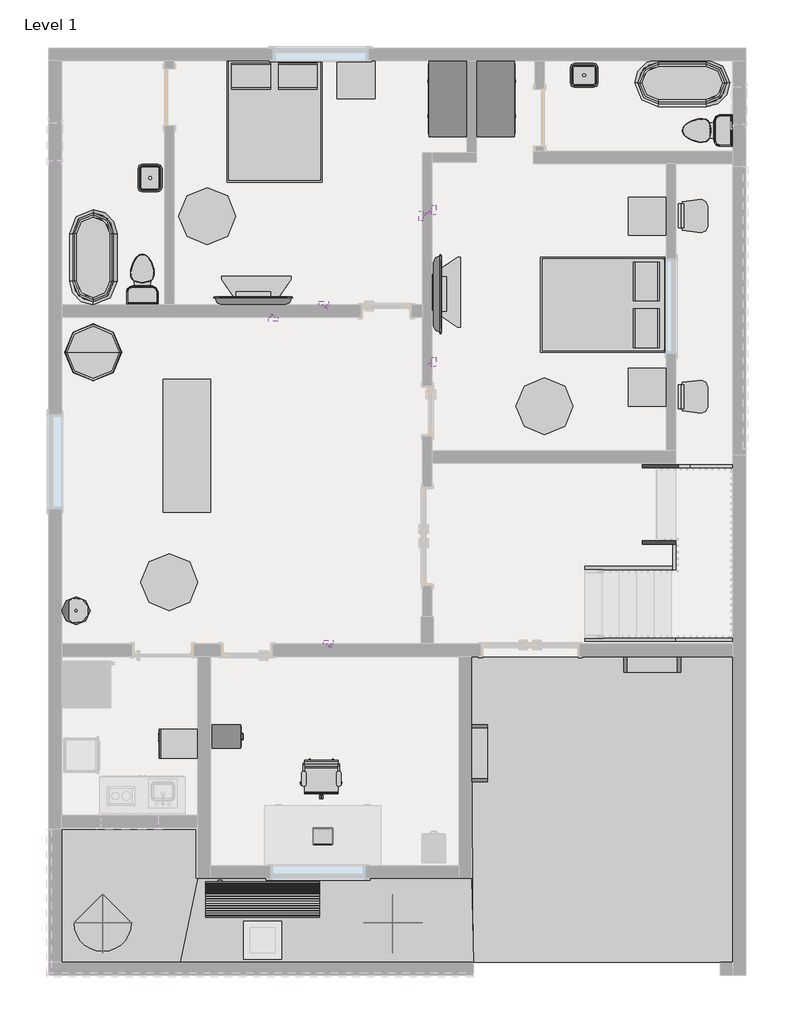
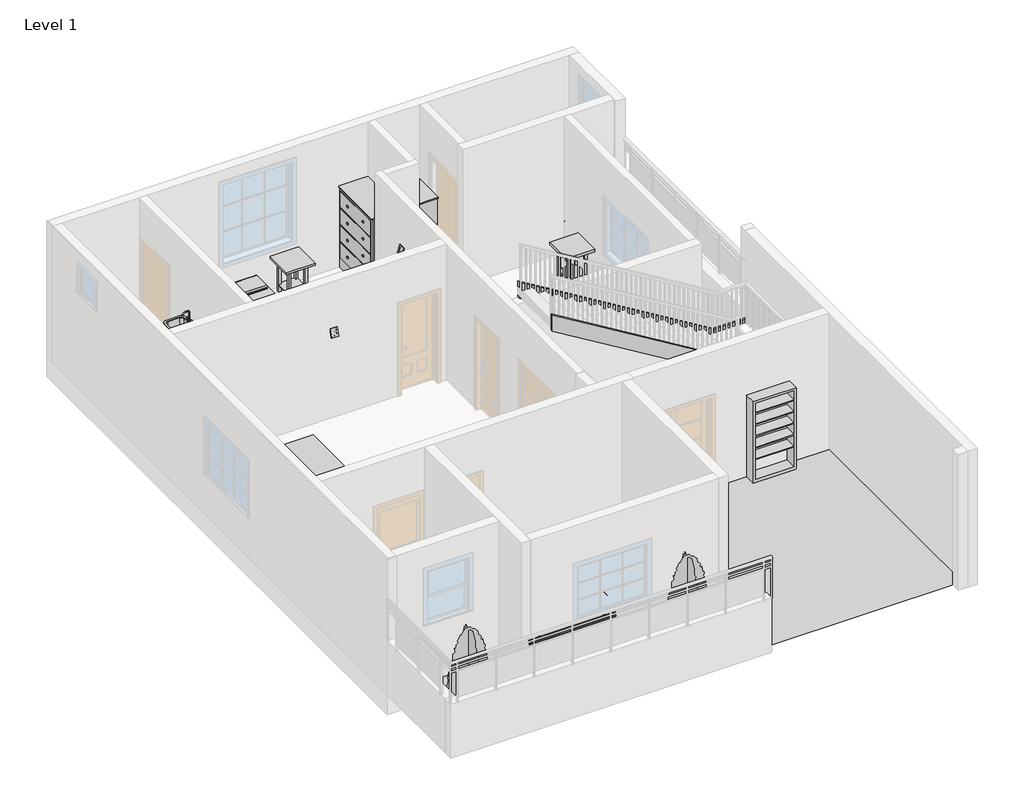
# One storey, part 4 of 4: 22 furniture elements, 11 proxies, 8 members, 7 flow terminals, 3 geographic elements.
"""IFC4 building model written with IfcOpenShell, lengths in millimetres."""

from ifc_helpers import new_model, si_unit, frame, origin, place, context, project, spatial, polyline, outline, extrude, faceted_brep, triangles, transform, mapped, element, save
from components import entourage_4c8cfd20, proxy_7e1014cc, rpc_picture_frame_rpc_picture_frame_c25e3fe9, flow_terminal_d49f872f, flow_terminal_62a433f7, toilet_domestic_3d_toilet_domestic_3d_f7549cf7, toilet_domestic_3d_toilet_domestic_3d_183bbd19, flow_terminal_b374fae2, furniture_1d2926bd, furniture_d4d3357e, chair_desk_chair_desk_ccc35c8f, chair_task_arms_chair_task_arms_fa5a08ef, furniture_9fa109b2, furniture_417d203a, furniture_fdf74506, tv_stand_tv_stand_6ce107e5, furniture_92191dda, furniture_905aceb5, furniture_4bee3317, furniture_5bc9ed15, furniture_c80d6d9c, geographic_element_235d1464, rpc_tree_conifer_chinese_juniper_7_1b9786cd

model = new_model("IFC4")

# Units and contexts
model_context = context("Model", 3, world=origin())
ifc_project = project(units=[si_unit("LENGTHUNIT", "METRE", prefix="MILLI")], contexts=[model_context])

# Site, building, storey
site = spatial("IfcSite", under=ifc_project)
building = spatial("IfcBuilding", under=site)
storey = spatial("IfcBuildingStorey", under=building, Name="Level 1", Elevation=0.0)

# Proxies
placement = place(None, origin())
element("IfcBuildingElementProxy", 1, Name="Building Element Proxy", at=placement, inside=storey, context=model_context, shape_type="Tessellation", body=[
    triangles([(-4983.3888428, 2180.3574657, 0.0), (-792.3886248, 2180.3574657, 0.0), (-792.3886248, -2721.8425827, 0.0), (-4957.988649, -2721.8425827, 0.0)], [[1, 4, 2], [3, 2, 4]], closed=False),
])
element("IfcBuildingElementProxy", 2, Name="Building Element Proxy", at=placement, inside=storey, context=model_context, shape_type="Tessellation", body=[
    triangles([(-11561.9884552, -588.24251, 0.0), (-9377.588649, -562.8424979, 0.0), (-9377.588649, -1375.6424858, 0.0), (-11561.9884552, -2721.8425827, 0.0), (-9661.5468979, -2721.8425827, 0.0)], [[1, 4, 3], [3, 2, 1], [3, 4, 5]], closed=False),
])
element("IfcBuildingElementProxy", 3, Name="Building Element Proxy", at=placement, inside=storey, context=model_context, shape_type="Tessellation", body=[
    triangles([(-9657.6913193, -2721.8425827, 0.0), (-9377.588649, -1375.6424858, 0.0), (-4983.3888428, -1375.6424858, 0.0), (-4957.988649, -2721.8425827, 0.0)], [[2, 1, 4], [4, 3, 2]], closed=False),
])
entourage_shape = entourage_4c8cfd20(model_context)
element("IfcBuildingElementProxy", 4, Name="Entourage", at=placement, inside=storey, context=model_context, shape_type="MappedRepresentation", body=[
    mapped(entourage_shape, transform((-7370.5830981, -664.4425054, 762.0), x_axis=(1.0, 0.0, 0.0), y_axis=(0.0, 1.0, 0.0), z_axis=(0.0, 0.0, 1.0))),
])
proxy_shape = proxy_7e1014cc(model_context)
element("IfcBuildingElementProxy", 5, Name="18\" x 24\" x 34 1/2\"", ObjectType="18\" x 24\" x 34 1/2\"", at=placement, inside=storey, context=model_context, shape_type="MappedRepresentation", body=[
    mapped(proxy_shape, transform((-9948.8381931, 1089.4749631, 0.0), x_axis=(0.0, -1.0, 0.0), y_axis=(1.0, 0.0, 0.0), z_axis=(0.0, 0.0, 1.0))),
])
rpc_picture_frame_rpc_picture_frame_shape = rpc_picture_frame_rpc_picture_frame_c25e3fe9(model_context)
element("IfcBuildingElementProxy", 6, Name="RPC Picture Frame : RPC Picture Frame", ObjectType="RPC Picture Frame : RPC Picture Frame", at=placement, inside=storey, context=model_context, shape_type="MappedRepresentation", body=[
    mapped(rpc_picture_frame_rpc_picture_frame_shape, transform((-7352.9458894, 7819.1574946, 1828.8), x_axis=(-0.9999999999999998, 0.0, 0.0), y_axis=(0.0, -0.9999999999999998, 0.0), z_axis=(0.0, 0.0, 1.0))),
])
element("IfcBuildingElementProxy", 7, Name="RPC Picture Frame : RPC Picture Frame", ObjectType="RPC Picture Frame : RPC Picture Frame", at=placement, inside=storey, context=model_context, shape_type="MappedRepresentation", body=[
    mapped(rpc_picture_frame_rpc_picture_frame_shape, transform((-5770.7886283, 9241.5574946, 1828.8), x_axis=(0.0, -1.0000000000000002, 0.0), y_axis=(1.0000000000000002, 0.0, 0.0), z_axis=(0.0, 0.0, 1.0))),
])
element("IfcBuildingElementProxy", 8, Name="RPC Picture Frame : RPC Picture Frame", ObjectType="RPC Picture Frame : RPC Picture Frame", at=placement, inside=storey, context=model_context, shape_type="MappedRepresentation", body=[
    mapped(rpc_picture_frame_rpc_picture_frame_shape, transform((-5618.3886283, 9336.9494679, 1828.8), x_axis=(0.0, 1.0000000000000004, 0.0), y_axis=(-1.0000000000000004, 0.0, 0.0), z_axis=(0.0, 0.0, 1.0))),
])
element("IfcBuildingElementProxy", 9, Name="RPC Picture Frame : RPC Picture Frame", ObjectType="RPC Picture Frame : RPC Picture Frame", at=placement, inside=storey, context=model_context, shape_type="MappedRepresentation", body=[
    mapped(rpc_picture_frame_rpc_picture_frame_shape, transform((-5618.3886283, 6905.8954271, 1828.8), x_axis=(0.0, 1.0000000000000002, 0.0), y_axis=(-1.0000000000000002, 0.0, 0.0), z_axis=(0.0, 0.0, 1.0))),
])
element("IfcBuildingElementProxy", 10, Name="RPC Picture Frame : RPC Picture Frame", ObjectType="RPC Picture Frame : RPC Picture Frame", at=placement, inside=storey, context=model_context, shape_type="MappedRepresentation", body=[
    mapped(rpc_picture_frame_rpc_picture_frame_shape, transform((-7281.3925432, 2383.5574946, 1828.8), x_axis=(-1.0, 0.0, 0.0), y_axis=(0.0, -1.0, 0.0), z_axis=(0.0, 0.0, 1.0))),
])
element("IfcBuildingElementProxy", 11, Name="RPC Picture Frame : RPC Picture Frame", ObjectType="RPC Picture Frame : RPC Picture Frame", at=placement, inside=storey, context=model_context, shape_type="MappedRepresentation", body=[
    mapped(rpc_picture_frame_rpc_picture_frame_shape, transform((-8165.6222602, 7615.9574946, 1828.8), x_axis=(1.0000000000000002, 0.0, 0.0), y_axis=(0.0, 1.0000000000000002, 0.0), z_axis=(0.0, 0.0, 1.0))),
])

# Flow terminals
flow_terminal_shape = flow_terminal_d49f872f(model_context)
element("IfcFlowTerminal", 12, ObjectType="Sink Vanity-Round : 19\" x 19\"", at=placement, inside=storey, context=model_context, shape_type="MappedRepresentation", body=[
    mapped(flow_terminal_shape, transform((-11245.3762507, 2820.305754, 457.2), x_axis=(0.0, 1.0000000000000002, 0.0), y_axis=(-1.0000000000000002, 0.0, 0.0), z_axis=(0.0, 0.0, 1.0))),
])
flow_terminal_2_shape = flow_terminal_62a433f7(model_context)
element("IfcFlowTerminal", 13, ObjectType="Sink Vanity-Square : 20\" x 18\"", at=placement, inside=storey, context=model_context, shape_type="MappedRepresentation", body=[
    mapped(flow_terminal_2_shape, transform((-3195.6778689, 11550.6120935, 609.6), x_axis=(1.0, 0.0, 0.0), y_axis=(0.0, 1.0, 0.0), z_axis=(0.0, 0.0, 1.0))),
])
element("IfcFlowTerminal", 14, ObjectType="Sink Vanity-Square : 20\" x 18\"", at=placement, inside=storey, context=model_context, shape_type="MappedRepresentation", body=[
    mapped(flow_terminal_2_shape, transform((-10091.1340294, 9866.8467351, 609.6), x_axis=(0.0, -1.0, 0.0), y_axis=(1.0, 0.0, 0.0), z_axis=(0.0, 0.0, 1.0))),
])
toilet_domestic_3d_toilet_domestic_3d_shape = toilet_domestic_3d_toilet_domestic_3d_f7549cf7(model_context)
toilet_domestic_3d_toilet_domestic_3d_2_shape = toilet_domestic_3d_toilet_domestic_3d_183bbd19(model_context)
element("IfcFlowTerminal", 15, ObjectType="Toilet-Domestic-3D : Toilet-Domestic-3D", at=placement, inside=storey, context=model_context, shape_type="MappedRepresentation", body=[
    mapped(toilet_domestic_3d_toilet_domestic_3d_shape, transform((-1300.3886283, 10613.1574946, 0.0), x_axis=(0.0, -1.0000000000000002, 0.0), y_axis=(1.0000000000000002, 0.0, 0.0), z_axis=(0.0, 0.0, 1.0))),
    mapped(toilet_domestic_3d_toilet_domestic_3d_2_shape, transform((-1300.3886283, 10613.1574946, 0.0), x_axis=(0.0, -1.0000000000000002, 0.0), y_axis=(1.0000000000000002, 0.0, 0.0), z_axis=(0.0, 0.0, 1.0))),
])
element("IfcFlowTerminal", 16, ObjectType="Toilet-Domestic-3D : Toilet-Domestic-3D", at=placement, inside=storey, context=model_context, shape_type="MappedRepresentation", body=[
    mapped(toilet_domestic_3d_toilet_domestic_3d_shape, transform((-10266.5886283, 8327.1574946, 0.0), x_axis=(-0.9999999999999998, 0.0, 0.0), y_axis=(0.0, -0.9999999999999998, 0.0), z_axis=(0.0, 0.0, 1.0))),
    mapped(toilet_domestic_3d_toilet_domestic_3d_2_shape, transform((-10266.5886283, 8327.1574946, 0.0), x_axis=(-0.9999999999999998, 0.0, 0.0), y_axis=(0.0, -0.9999999999999998, 0.0), z_axis=(0.0, 0.0, 1.0))),
])
flow_terminal_3_shape = flow_terminal_b374fae2(model_context)
element("IfcFlowTerminal", 17, ObjectType="Tub-Free Standing-3D : 30\" x 60\"", at=placement, inside=storey, context=model_context, shape_type="MappedRepresentation", body=[
    mapped(flow_terminal_3_shape, transform((-1605.1886283, 11375.1574946, 0.0), x_axis=(0.0, -1.0, 0.0), y_axis=(1.0, 0.0, 0.0), z_axis=(0.0, 0.0, 1.0))),
])
element("IfcFlowTerminal", 18, ObjectType="Tub-Free Standing-3D : 30\" x 60\"", at=placement, inside=storey, context=model_context, shape_type="MappedRepresentation", body=[
    mapped(flow_terminal_3_shape, transform((-11053.9886283, 8581.1574946, 0.0), x_axis=(-1.0000000000000002, 0.0, 0.0), y_axis=(0.0, -1.0000000000000002, 0.0), z_axis=(0.0, 0.0, 1.0))),
])

# Furniture
furniture_shape = furniture_1d2926bd(model_context)
element("IfcFurniture", 19, ObjectType="Bed-Box : Queen 60\" x 79\"", at=placement, inside=storey, context=model_context, shape_type="MappedRepresentation", body=[
    mapped(furniture_shape, transform((-2640.7591201, 8158.3099536, 0.0), x_axis=(0.0, -1.0, 0.0), y_axis=(1.0, 0.0, 0.0), z_axis=(0.0, 0.0, 1.0))),
])
element("IfcFurniture", 20, ObjectType="Bed-Box : Queen 60\" x 79\"", at=placement, inside=storey, context=model_context, shape_type="MappedRepresentation", body=[
    mapped(furniture_shape, transform((-8484.8410873, 11025.3870028, 0.0), x_axis=(1.0, 0.0, 0.0), y_axis=(0.0, 1.0, 0.0), z_axis=(0.0, 0.0, 1.0))),
])
furniture_2_shape = furniture_d4d3357e(model_context)
element("IfcFurniture", 21, ObjectType="Cabinet-File 5 Drawer : 15\" x 18\"", at=placement, inside=storey, context=model_context, shape_type="MappedRepresentation", body=[
    mapped(furniture_2_shape, transform((-9062.5229284, 1025.5539416, 0.0), x_axis=(0.0, 1.0, 0.0), y_axis=(-1.0, 0.0, 0.0), z_axis=(0.0, 0.0, 1.0))),
])
chair_desk_chair_desk_shape = chair_desk_chair_desk_ccc35c8f(model_context)
element("IfcFurniture", 22, ObjectType="Chair-Desk : Chair-Desk", at=placement, inside=storey, context=model_context, shape_type="MappedRepresentation", body=[
    mapped(chair_desk_chair_desk_shape, transform((-1605.1886283, 6345.9574946, 0.0), x_axis=(0.0, -1.0000000000000007, 0.0), y_axis=(1.0000000000000007, 0.0, 0.0), z_axis=(0.0, 0.0, 1.0))),
])
element("IfcFurniture", 23, ObjectType="Chair-Desk : Chair-Desk", at=placement, inside=storey, context=model_context, shape_type="MappedRepresentation", body=[
    mapped(chair_desk_chair_desk_shape, transform((-1605.1886283, 9241.5574946, 0.0), x_axis=(0.0, -1.0000000000000002, 0.0), y_axis=(1.0000000000000002, 0.0, 0.0), z_axis=(0.0, 0.0, 1.0))),
])
chair_task_arms_chair_task_arms_shape = chair_task_arms_chair_task_arms_fa5a08ef(model_context)
element("IfcFurniture", 24, ObjectType="Chair-Task Arms : Chair-Task Arms", at=placement, inside=storey, context=model_context, shape_type="MappedRepresentation", body=[
    mapped(chair_task_arms_chair_task_arms_shape, transform((-7255.3978086, 268.9033962, 0.0), x_axis=(-0.9999999999999999, 0.0, 0.0), y_axis=(0.0, -0.9999999999999999, 0.0), z_axis=(0.0, 0.0, 1.0))),
])
furniture_3_shape = furniture_9fa109b2(model_context)
element("IfcFurniture", 25, ObjectType="Dresser : 48\" x 72\" x 24\"", at=placement, inside=storey, context=model_context, shape_type="MappedRepresentation", body=[
    mapped(furniture_3_shape, transform((-4965.5515824, 11390.3507544, 0.0), x_axis=(0.0, 1.0, 0.0), y_axis=(-1.0, 0.0, 0.0), z_axis=(0.0, 0.0, 1.0))),
])
element("IfcFurniture", 26, ObjectType="Dresser : 48\" x 72\" x 24\"", at=placement, inside=storey, context=model_context, shape_type="MappedRepresentation", body=[
    mapped(furniture_3_shape, transform((-5001.2256742, 10851.9642347, 0.0), x_axis=(0.0, -1.0000000000000007, 0.0), y_axis=(1.0000000000000007, 0.0, 0.0), z_axis=(0.0, 0.0, 1.0))),
])
furniture_4_shape = furniture_417d203a(model_context)
element("IfcFurniture", 27, ObjectType="Shelving : 36\" x 10\" x 72\"", at=placement, inside=storey, context=model_context, shape_type="MappedRepresentation", body=[
    mapped(furniture_4_shape, transform((-5161.1886283, 630.9574946, 0.0), x_axis=(0.0, 1.0, 0.0), y_axis=(-1.0, 0.0, 0.0), z_axis=(0.0, 0.0, 1.0))),
])
element("IfcFurniture", 28, ObjectType="Shelving : 36\" x 10\" x 72\"", at=placement, inside=storey, context=model_context, shape_type="MappedRepresentation", body=[
    mapped(furniture_4_shape, transform((-2087.7886283, 1748.5574946, 0.0), x_axis=(-1.0000000000000002, 0.0, 0.0), y_axis=(0.0, -1.0000000000000002, 0.0), z_axis=(0.0, 0.0, 1.0))),
])
furniture_5_shape = furniture_fdf74506(model_context)
element("IfcFurniture", 29, ObjectType="TV - Flat Screen : 50\"", at=placement, inside=storey, context=model_context, shape_type="MappedRepresentation", body=[
    mapped(furniture_5_shape, transform((-8492.5331425, 7877.6961182, 914.4), x_axis=(-1.0000000000000002, 0.0, 0.0), y_axis=(0.0, -1.0000000000000002, 0.0), z_axis=(0.0, 0.0, 1.0))),
])
element("IfcFurniture", 30, ObjectType="TV - Flat Screen : 50\"", at=placement, inside=storey, context=model_context, shape_type="MappedRepresentation", body=[
    mapped(furniture_5_shape, transform((-5539.8500047, 7993.819929, 914.4), x_axis=(0.0, 1.0000000000000002, 0.0), y_axis=(-1.0000000000000002, 0.0, 0.0), z_axis=(0.0, 0.0, 1.0))),
])
tv_stand_tv_stand_shape = tv_stand_tv_stand_6ce107e5(model_context)
element("IfcFurniture", 31, ObjectType="TV Stand : TV Stand", at=placement, inside=storey, context=model_context, shape_type="MappedRepresentation", body=[
    mapped(tv_stand_tv_stand_shape, transform((-8312.6006262, 7819.1574946, 0.0), x_axis=(-1.0000000000000002, 0.0, 0.0), y_axis=(0.0, -1.0000000000000002, 0.0), z_axis=(0.0, 0.0, 1.0))),
])
element("IfcFurniture", 32, ObjectType="TV Stand : TV Stand", at=placement, inside=storey, context=model_context, shape_type="MappedRepresentation", body=[
    mapped(tv_stand_tv_stand_shape, transform((-5618.3886283, 7897.1694925, 0.0), x_axis=(0.0, 1.0, 0.0), y_axis=(-1.0, 0.0, 0.0), z_axis=(0.0, 0.0, 1.0))),
])
furniture_6_shape = furniture_92191dda(model_context)
element("IfcFurniture", 33, ObjectType="Table-Dining : 30\" x 84\" x 22\"", at=placement, inside=storey, context=model_context, shape_type="MappedRepresentation", body=[
    mapped(furniture_6_shape, transform((-9460.1775505, 5540.2917279, 0.0), x_axis=(0.0, 1.0, 0.0), y_axis=(-1.0, 0.0, 0.0), z_axis=(0.0, 0.0, 1.0))),
])
furniture_7_shape = furniture_905aceb5(model_context)
element("IfcFurniture", 34, ObjectType="Table-Dining Round w Chairs : 36\" Diameter", at=placement, inside=storey, context=model_context, shape_type="MappedRepresentation", body=[
    mapped(furniture_7_shape, transform((-9938.4705955, 3559.0361831, 0.0), x_axis=(1.0, 0.0, 0.0), y_axis=(0.0, 1.0, 0.0), z_axis=(0.0, 0.0, 1.0))),
])
furniture_8_shape = furniture_4bee3317(model_context)
element("IfcFurniture", 35, ObjectType="Table-Ellipse : 72\" x 36\"", at=placement, inside=storey, context=model_context, shape_type="MappedRepresentation", body=[
    mapped(furniture_8_shape, transform((-9225.1886283, 9241.5574946, 0.0), x_axis=(0.0, 0.9999999999999998, 0.0), y_axis=(-0.9999999999999998, 0.0, 0.0), z_axis=(0.0, 0.0, 1.0))),
])
element("IfcFurniture", 36, ObjectType="Table-Ellipse : 72\" x 36\"", at=placement, inside=storey, context=model_context, shape_type="MappedRepresentation", body=[
    mapped(furniture_8_shape, transform((-3814.9886283, 6193.5574946, 0.0), x_axis=(-1.0000000000000002, 0.0, 0.0), y_axis=(0.0, -1.0000000000000002, 0.0), z_axis=(0.0, 0.0, 1.0))),
])
furniture_9_shape = furniture_5bc9ed15(model_context)
element("IfcFurniture", 37, ObjectType="Table-Night Stand : 24\" x 24\" x 30\"", at=placement, inside=storey, context=model_context, shape_type="MappedRepresentation", body=[
    mapped(furniture_9_shape, transform((-2472.5222586, 8936.7574946, 0.0), x_axis=(1.0, 0.0, 0.0), y_axis=(0.0, 1.0, 0.0), z_axis=(0.0, 0.0, 1.0))),
])
element("IfcFurniture", 38, ObjectType="Table-Night Stand : 24\" x 24\" x 30\"", at=placement, inside=storey, context=model_context, shape_type="MappedRepresentation", body=[
    mapped(furniture_9_shape, transform((-2472.5222586, 6193.5574946, 0.0), x_axis=(1.0, 0.0, 0.0), y_axis=(0.0, 1.0, 0.0), z_axis=(0.0, 0.0, 1.0))),
])
element("IfcFurniture", 39, ObjectType="Table-Night Stand : 24\" x 24\" x 30\"", at=placement, inside=storey, context=model_context, shape_type="MappedRepresentation", body=[
    mapped(furniture_9_shape, transform((-7146.1222586, 11121.1574946, 0.0), x_axis=(1.0, 0.0, 0.0), y_axis=(0.0, 1.0, 0.0), z_axis=(0.0, 0.0, 1.0))),
])
furniture_10_shape = furniture_c80d6d9c(model_context)
element("IfcFurniture", 40, ObjectType="Table-Round : 36\" Diameter", at=placement, inside=storey, context=model_context, shape_type="MappedRepresentation", body=[
    mapped(furniture_10_shape, transform((-11053.9886283, 7057.1574946, 0.0), x_axis=(1.0, 0.0, 0.0), y_axis=(0.0, 1.0, 0.0), z_axis=(0.0, 0.0, 1.0))),
])

# Geographic elements
geographic_element_shape = geographic_element_235d1464(model_context)
element("IfcGeographicElement", 41, ObjectType="Park Bench : 72\"", at=placement, inside=storey, context=model_context, shape_type="MappedRepresentation", body=[
    mapped(geographic_element_shape, transform((-8336.1886283, -1680.4425054, 0.0), x_axis=(1.0, 0.0, 0.0), y_axis=(0.0, 1.0, 0.0), z_axis=(0.0, 0.0, 1.0))),
])
rpc_tree_conifer_chinese_juniper_7_shape = rpc_tree_conifer_chinese_juniper_7_1b9786cd(model_context)
element("IfcGeographicElement", 42, ObjectType="RPC Tree - Conifer : Chinese Juniper - 7'", at=placement, inside=storey, context=model_context, shape_type="MappedRepresentation", body=[
    mapped(rpc_tree_conifer_chinese_juniper_7_shape, transform((-10901.7852994, -2086.8425054, 0.0), x_axis=(1.0, 0.0, 0.0), y_axis=(0.0, 1.0, 0.0), z_axis=(0.0, 0.0, 1.0))),
])
element("IfcGeographicElement", 43, ObjectType="RPC Tree - Conifer : Chinese Juniper - 7'", at=placement, inside=storey, context=model_context, shape_type="MappedRepresentation", body=[
    mapped(rpc_tree_conifer_chinese_juniper_7_shape, transform((-6253.5852994, -2086.8425054, 0.0), x_axis=(1.0, 0.0, 0.0), y_axis=(0.0, 1.0, 0.0), z_axis=(0.0, 0.0, 1.0))),
])

# Members
element("IfcMember", 44, ObjectType="Stringer - 2\" Width", at=placement, inside=storey, context=model_context, shape_type="SweptSolid", body=[
    extrude(outline(polyline([(212.114512, -3170.5888787), (0.0, -3170.5888787), (0.0, -2932.5033669), (712.0695386, -1757.5886283), (1068.4783001, -1757.5886283), (212.114512, -3170.5888787)])), frame((0.0, 3576.1973029, 0.0), z_axis=(0.0, 1.0, 0.0), x_axis=(0.0, 0.0, 1.0)), (0.0, 0.0, 1.0), 50.8),
])
element("IfcMember", 45, ObjectType="Stringer - 2\" Width", at=placement, inside=storey, context=model_context, shape_type="SweptSolid", body=[
    extrude(outline(polyline([(212.114512, -3170.5888787), (0.0, -3170.5888787), (0.0, -2932.5033669), (787.4, -1633.2933669), (1092.2, -1718.4478234), (212.114512, -3170.5888787)])), frame((0.0, 2424.0939653, 0.0), z_axis=(0.0, 1.0, 0.0), x_axis=(0.0, 0.0, 1.0)), (0.0, 0.0, 1.0), 50.8),
])
element("IfcMember", 46, ObjectType="Stringer - 2\" Width", at=placement, inside=storey, context=model_context, shape_type="SweptSolid", body=[
    extrude(outline(polyline([(871.7057504, -1706.7886283), (1228.114512, -1706.7886283), (3598.7811786, -5618.3886283), (3242.3724171, -5618.3886283), (871.7057504, -1706.7886283)])), frame((0.0, 3983.7574946, 0.0), z_axis=(0.0, 1.0, 0.0), x_axis=(0.0, 0.0, 1.0)), (0.0, 0.0, 1.0), 50.8),
])
element("IfcMember", 47, ObjectType="Stringer - 2\" Width", at=placement, inside=storey, context=model_context, shape_type="SweptSolid", body=[
    extrude(outline(polyline([(787.4, -1567.6841401), (1092.2, -1482.5296836), (3598.7811786, -5618.3886283), (3242.3724171, -5618.3886283), (787.4, -1567.6841401)])), frame((0.0, 5206.8078573, 0.0), z_axis=(0.0, 1.0, 0.0), x_axis=(0.0, 0.0, 1.0)), (0.0, 0.0, 1.0), 50.8),
])
element("IfcMember", 48, ObjectType="Stringer - 2\" Width", at=placement, inside=storey, context=model_context, shape_type="SweptSolid", body=[
    extrude(outline(polyline([(-1757.5886283, 3983.7574946), (-1706.7886283, 3983.7574946), (-1706.7886283, 3576.1973029), (-1757.5886283, 3576.1973029), (-1757.5886283, 3983.7574946)])), frame((0.0, 0.0, 787.4), z_axis=(0.0, 0.0, 1.0), x_axis=(1.0, 0.0, 0.0)), (0.0, 0.0, 1.0), 304.8),
])
element("IfcMember", 49, ObjectType="Stringer - 2\" Width", at=placement, inside=storey, context=model_context, shape_type="Brep", body=[
    faceted_brep([(-1718.4478234, 2474.8939653, 1092.2), (-1718.4478234, 2424.0939653, 1092.2), (-741.5886283, 2424.0939653, 1092.2), (-792.3886283, 2474.8939653, 1092.2), (-1633.2933669, 2474.8939653, 787.4), (-792.3886283, 2474.8939653, 787.4), (-1633.2933669, 2424.0939653, 787.4), (-741.5886283, 2424.0939653, 787.4)], [[[0, 1, 2, 3]], [[4, 0, 3, 5]], [[6, 4, 5, 7]], [[1, 6, 7, 2]], [[1, 0, 4, 6]], [[2, 7, 5, 3]]]),
])
element("IfcMember", 50, ObjectType="Stringer - 2\" Width", at=placement, inside=storey, context=model_context, shape_type="SweptSolid", body=[
    extrude(outline(polyline([(-741.5886283, 2424.0939653), (-792.3886283, 2474.8939653), (-792.3886283, 5206.8078573), (-741.5886283, 5257.6078573), (-741.5886283, 2424.0939653)])), frame((0.0, 0.0, 787.4), z_axis=(0.0, 0.0, 1.0), x_axis=(1.0, 0.0, 0.0)), (0.0, 0.0, 1.0), 304.8),
])
element("IfcMember", 51, ObjectType="Stringer - 2\" Width", at=placement, inside=storey, context=model_context, shape_type="Brep", body=[
    faceted_brep([(-792.3886283, 5206.8078573, 1092.2), (-741.5886283, 5257.6078573, 1092.2), (-1482.5296836, 5257.6078573, 1092.2), (-1482.5296836, 5206.8078573, 1092.2), (-792.3886283, 5206.8078573, 787.4), (-1567.6841401, 5206.8078573, 787.4), (-741.5886283, 5257.6078573, 787.4), (-1567.6841401, 5257.6078573, 787.4)], [[[0, 1, 2, 3]], [[4, 0, 3, 5]], [[6, 4, 5, 7]], [[1, 6, 7, 2]], [[1, 0, 4, 6]], [[2, 7, 5, 3]]]),
])

save(model, "model.ifc")

# Revit data of these elements
# Type
#   built-in parameter 1005195 = "RPC-16-N04H-AQSP-D1N4-43SU-6GKQ-C3KU-1C"
#   Height = 0
# Type "18\" x 24\" x 34 1/2\""
#   Label = "T"
#   Assembly Code = "E1090400"
#   Depth = 2' - 0"
#   Height = 2' - 10 1/2"
#   Width = 1' - 6"
#   Panel Face Material = Plastic, Opaque Black
#   Trach Compact. Material = Steel, Paint Finish, Ivory, Matte
#   Default Elevation = 0
# Type "RPC Picture Frame : RPC Picture Frame"
#   built-in parameter 1005198 = "{2, 15},{39, RPC-16-8M5E-0H3T-F0AH-3U0K-JLQ7-G28B-AU},{1, 0},{1, 0},{2, 19},{1, 8},{5, Color},{1, 0},{1, 0},{3, 0.8},{3, 0.8},{3, 0.8},{1, 8},{7, BBoxMin},{1, 0},{1, 0},{1, 0},{1, 0},{1, 0},{1, 8},{7, BBoxMax},{1, 0},{1, 0},{1, 0},{1, 0},{1, 0},{2, 11},{9, RPCTypeId},{1, 0},{1, 0},{39, RPC-16-8M5E-0H3T-F0AH-3U0K-JLQ7-G28B-AU},{1, 6},{14, RPCPlantHeight},{1, 0},{1, 0},{5, 0.625},{2, 11},{7, keyword},{1, 0},{1, 0},{33, :RPCs:Office Clutter:Geometry:RPC},{2, 11},{8, category},{1, 0},{1, 0},{14, Office Clutter},{2, 11},{12, LocalizedUID},{1, 0},{1, 0},{13, Picture Frame},{2, 14},{6, Height},{1, 0},{1, 0},{5, 0.625},{1, 2},{16, Cast Reflections},{1, 0},{1, 0},{1, 0},{1, 2},{8, Portrait},{1, 0},{1, 0},{1, 1},{1, 2},{5, Stand},{1, 0},{1, 0},{1, 1},{2, 11},{10, RPCL_Frame},{1, 0},{1, 0},{5, Frame},{1, 4},{14, Frame Material},{1, 0},{1, 0},{1, 0},{2, 11},{12, RPCL_Picture},{1, 0},{1, 0},{7, Picture},{2, 11},{15, Picture Preview},{1, 0},{1, 0},{65, __RPC:/object data/textures/object/Photo/Photo0/textures/Portrait},{2, 11},{17, i_Picture Preview},{1, 0},{1, 0},{0, },{1, 2},{18, Use Custom Picture},{1, 0},{1, 0},{1, 0},{2, 11},{17, Picture File Name},{1, 0},{1, 0},{0, },{21, assetlibrary_base.fbx},{1, 5},"
#   built-in parameter 1005195 = "RPC-16-8M5E-0H3T-F0AH-3U0K-JLQ7-G28B-AU"
#   Height = 0
# Type "Sink Vanity-Round : 19\" x 19\""
#   Assembly Code = "D2010400"
#   Top Of Counter = 2' - 7"
#   Basin Material = Porcelain, Linen
#   Faucet Material = Steel, Polished
#   Default Elevation = 0
# Type "Sink Vanity-Square : 20\" x 18\""
#   Assembly Code = "D2010400"
#   Counter Height = 2' - 7"
#   Depth = 1' - 6"
#   Width = 1' - 8"
#   Basin Material = Porcelain, Linen
#   Faucet Material = Steel, Polished
#   Default Elevation = 0
# Type "Toilet-Domestic-3D : Toilet-Domestic-3D"
#   Assembly Code = "D2010110"
#   Toilet - Bowl/Basin Material = Porcelain, Linen
#   Toilet - Seat Material = Laminate, Linen, Matte
#   Default Elevation = 0
# Type "Tub-Free Standing-3D : 30\" x 60\""
#   Assembly Code = "D2010110"
#   Height = 1' - 6"
#   Length = 5' - 0"
#   Width = 2' - 6"
#   Tub Material = Porcelain, Ivory
#   Default Elevation = 0
# Type "Bed-Box : Queen 60\" x 79\""
#   Assembly Code = "E2020200"
#   Length = 6' - 7"
#   Width = 5' - 0"
#   Frame Material = Birch
#   Mattress Material = Linen, White
#   Default Elevation = 0
# Type "Cabinet-File 5 Drawer : 15\" x 18\""
#   Assembly Code = "E2020200"
#   Depth = 1' - 6"
#   Height = 5' - 0"
#   Width = 1' - 3"
#   Cabinet Material = Steel, Paint Finish, Ivory, Glossy
#   Handle Material = Steel, Chrome Plated
#   Default Elevation = 0
# Type "Chair-Desk : Chair-Desk"
#   Assembly Code = "E2020200"
#   Seat/Back Material = Textile - Slate Blue
#   Base Material = Steel, Chrome Plated
#   Default Elevation = 0
# Type "Chair-Task Arms : Chair-Task Arms"
#   Assembly Code = "E2020200"
#   Base Material = Plastic, Opaque Black
#   Caster Material = Plastic, Opaque Black
#   Seat/Back Material = Textile - Slate Blue
#   Default Elevation = 0
# Type "Dresser : 48\" x 72\" x 24\""
#   Assembly Code = "E2020200"
#   Depth = 2' - 0"
#   Height = 6' - 0"
#   Width = 4' - 0"
#   Dresser Material = Laminate - Ivory, Glossy
#   Drawer Material = Laminate, Ivory, Matte
#   Knob Material = Cherry
#   Default Elevation = 0
# Type "Shelving : 36\" x 10\" x 72\""
#   Assembly Code = "E2020200"
#   Depth = 0' - 10"
#   Height = 6' - 0"
#   Width = 3' - 0"
#   Shelving Unit Material = Birch
#   Default Elevation = 0
# Type "TV - Flat Screen : 50\""
#   SinAng = 0' - 0.0193"
#   L = 3' - 7.57782"
#   H = 2' - 0.51477"
#   Thickness = 0' - 4.33071"
#   Diagonal = 4' - 2"
#   CosAng = 0' - 0.03431"
#   Stand [instance default] = yes
#   Default Elevation = 0
# Type "TV Stand : TV Stand"
#   Depth = 1' - 6"
#   Width = 3' - 8"
#   Height = 1' - 7 1/2"
#   Finish = Melamine - Gray
#   Default Elevation = 0
# Type "Table-Dining : 30\" x 84\" x 22\""
#   Assembly Code = "E2020200"
#   Height = 1' - 10"
#   Length = 7' - 0"
#   Width = 2' - 6"
#   Base Material = Steel, Chrome Plated
#   Top Material = Glass - Clear, Grey
#   Default Elevation = 0
# Type "Table-Dining Round w Chairs : 36\" Diameter"
#   Assembly Code = "E2020200"
#   Radius = 1' - 6"
#   Diameter = 3' - 0"
#   Height = 2' - 6"
#   Chairs = 4
#   Base Material = Pine
#   Top Material = Laminate, Linen, Matte
#   Default Elevation = 0
# Type "Table-Ellipse : 72\" x 36\""
#   Assembly Code = "E2020200"
#   Half Width = 1' - 6"
#   Half Length = 1' - 6"
#   Height = 2' - 6"
#   Length = 3' - 0"
#   Width = 3' - 0"
#   Base Material = Birch
#   Top Material = Laminate - Black
#   Default Elevation = 0
# Type "Table-Night Stand : 24\" x 24\" x 30\""
#   Assembly Code = "E2020200"
#   Depth = 2' - 0"
#   Height = 2' - 6"
#   Width = 2' - 0"
#   Base Material = Birch
#   Top Material = Laminate, Ivory, Matte
#   Default Elevation = 0
# Type "Table-Round : 36\" Diameter"
#   Assembly Code = "E2020200"
#   Base Radius = 0' - 10"
#   Height = 2' - 6"
#   Radius = 1' - 6"
#   Base Material = Steel, Chrome Plated
#   Top Material = Birch
#   Default Elevation = 0
# Type "Park Bench : 72\""
#   Length = 6' - 0"
#   Seat Material = Wood - Teak
#   Frame Material = Steel, Paint Finish, Dark Gray, Matte
# Type "RPC Tree - Conifer : Chinese Juniper - 7'"
#   built-in parameter 1005198 = "{2, 15},{39, RPC-16-FUM3-UUQ0-UBF0-N000-ST1L-LVER-AU},{1, 0},{1, 0},{2, 13},{1, 8},{5, Color},{1, 0},{1, 0},{3, 0.8},{3, 0.8},{3, 0.8},{1, 8},{7, BBoxMin},{1, 0},{1, 0},{1, 0},{1, 0},{1, 0},{1, 8},{7, BBoxMax},{1, 0},{1, 0},{1, 0},{1, 0},{1, 0},{2, 11},{9, RPCTypeId},{1, 0},{1, 0},{39, RPC-16-FUM3-UUQ0-UBF0-N000-ST1L-LVER-AU},{1, 6},{14, RPCPlantHeight},{1, 0},{1, 0},{1, 7},{2, 11},{7, keyword},{1, 0},{1, 0},{34, :RPCs:Trees [General]:Geometry:RPC},{2, 11},{8, category},{1, 0},{1, 0},{15, Trees [General]},{2, 11},{12, LocalizedUID},{1, 0},{1, 0},{15, Chinese Juniper},{2, 14},{6, Height},{1, 0},{1, 0},{1, 7},{1, 2},{16, Cast Reflections},{1, 0},{1, 0},{1, 0},{1, 2},{12, Cast Shadows},{1, 0},{1, 0},{1, 1},{1, 2},{9, Lock View},{1, 0},{1, 0},{1, 0},{1, 4},{5, ViewC},{1, 0},{1, 0},{1, 0},{21, assetlibrary_base.fbx},{1, 5},"
#   built-in parameter 1005195 = "RPC-16-FUM3-UUQ0-UBF0-N000-ST1L-LVER-AU"
#   Type Comments = "Chinese Juniper"
#   Assembly Code = "G2050500"
#   Height = 7' - 0"
#   Description = (empty or 0)
#   Default Elevation = 0
# Elements 1, 2, 3 (IfcBuildingElementProxy)
#   Material = none
#   Phase Created = New Construction
# Element 4 (IfcBuildingElementProxy)
#   Phase Created = New Construction
# Element 5 (IfcBuildingElementProxy, "18\" x 24\" x 34 1/2\"")
#   Phase Created = New Construction
#   Materials on its faces: "Steel, Paint Finish, Ivory, Matte", "Plastic, Opaque Black"
# Elements 6, 7, 8, 9, 10, 11 (IfcBuildingElementProxy, "RPC Picture Frame : RPC Picture Frame")
#   Phase Created = New Construction
# Element 12 (IfcFlowTerminal, "Sink Vanity-Round : 19\" x 19\"")
#   Mark = "8"
#   Phase Created = New Construction
#   Materials on its faces: "Porcelain, Linen", "Steel, Polished"
# Element 13 (IfcFlowTerminal, "Sink Vanity-Square : 20\" x 18\"")
#   Mark = "3"
#   Phase Created = New Construction
#   Materials on its faces: "Porcelain, Linen", "Steel, Polished"
# Element 14 (IfcFlowTerminal, "Sink Vanity-Square : 20\" x 18\"")
#   Mark = "4"
#   Phase Created = New Construction
#   Materials on its faces: "Porcelain, Linen", "Steel, Polished"
# Element 15 (IfcFlowTerminal, "Toilet-Domestic-3D : Toilet-Domestic-3D")
#   Mark = "2"
#   Phase Created = New Construction
#   Materials on its faces: "Porcelain, Linen", "Laminate, Linen, Matte"
# Element 16 (IfcFlowTerminal, "Toilet-Domestic-3D : Toilet-Domestic-3D")
#   Mark = "5"
#   Phase Created = New Construction
#   Materials on its faces: "Porcelain, Linen", "Laminate, Linen, Matte"
# Element 17 (IfcFlowTerminal, "Tub-Free Standing-3D : 30\" x 60\"")
#   Mark = "1"
#   Phase Created = New Construction
#   Materials on its faces: "Porcelain, Ivory"
# Element 18 (IfcFlowTerminal, "Tub-Free Standing-3D : 30\" x 60\"")
#   Mark = "6"
#   Phase Created = New Construction
#   Materials on its faces: "Porcelain, Ivory"
# Elements 19, 20 (IfcFurniture, "Bed-Box : Queen 60\" x 79\"")
#   Phase Created = New Construction
#   Materials on its faces: "Birch", "Linen, White"
# Element 21 (IfcFurniture, "Cabinet-File 5 Drawer : 15\" x 18\"")
#   Phase Created = New Construction
#   Materials on its faces: "Steel, Chrome Plated", "Steel, Paint Finish, Ivory, Glossy"
# Elements 22, 23 (IfcFurniture, "Chair-Desk : Chair-Desk")
#   Phase Created = New Construction
#   Materials on its faces: "Steel, Chrome Plated", "Textile - Slate Blue"
# Element 24 (IfcFurniture, "Chair-Task Arms : Chair-Task Arms")
#   Phase Created = New Construction
#   Materials on its faces: "Plastic, Opaque Black", "Textile - Slate Blue"
# Elements 25, 26 (IfcFurniture, "Dresser : 48\" x 72\" x 24\"")
#   Phase Created = New Construction
#   Materials on its faces: "Laminate, Ivory, Matte", "Cherry", "Laminate - Ivory, Glossy"
# Elements 27, 28 (IfcFurniture, "Shelving : 36\" x 10\" x 72\"")
#   Phase Created = New Construction
#   Materials on its faces: "Birch"
# Elements 29, 30 (IfcFurniture, "TV - Flat Screen : 50\"")
#   Stand = yes
#   Phase Created = New Construction
#   Materials on its faces: "TV - Black", "TV - Glass", "TV - Screen"
# Elements 31, 32 (IfcFurniture, "TV Stand : TV Stand")
#   Phase Created = New Construction
#   Materials on its faces: "Melamine - Gray", "Glass - Shelves"
# Element 33 (IfcFurniture, "Table-Dining : 30\" x 84\" x 22\"")
#   Phase Created = New Construction
#   Materials on its faces: "Steel, Chrome Plated", "Glass - Clear, Grey"
# Element 34 (IfcFurniture, "Table-Dining Round w Chairs : 36\" Diameter")
#   Phase Created = New Construction
#   Materials on its faces: "Pine", "Laminate, Linen, Matte"
# Elements 35, 36 (IfcFurniture, "Table-Ellipse : 72\" x 36\"")
#   Phase Created = New Construction
#   Materials on its faces: "Birch", "Laminate - Black"
# Elements 37, 38, 39 (IfcFurniture, "Table-Night Stand : 24\" x 24\" x 30\"")
#   Phase Created = New Construction
#   Materials on its faces: "Birch", "Laminate, Ivory, Matte"
# Element 40 (IfcFurniture, "Table-Round : 36\" Diameter")
#   Phase Created = New Construction
#   Materials on its faces: "Steel, Chrome Plated", "Birch"
# Element 41 (IfcGeographicElement, "Park Bench : 72\"")
#   Phase Created = New Construction
#   Materials on its faces: "Wood - Teak", "Steel, Paint Finish, Dark Gray, Matte"
# Elements 42, 43 (IfcGeographicElement, "RPC Tree - Conifer : Chinese Juniper - 7'")
#   Phase Created = New Construction
# Elements 44, 45, 46, 47, 48, 49, 50, 51 (IfcMember, "Stringer - 2\" Width")
#   Phase Created = New Construction
# Materials
#   "Plastic, Opaque Black": class "Plastic", colour RGB 0 0 0, transparency 0.7, Description = "Plastic, generic, opaque black", Cost = 0
#   "Steel, Paint Finish, Ivory, Matte": class "Metal", colour RGB 247 247 239, transparency 0, Description = "Steel, paint finish, ivory, matte", Cost = 0
#   "Porcelain, Linen": class "Ceramic", colour RGB 249 239 230, transparency 0, Description = "Porcelain, linen", Cost = 0
#   "Steel, Polished": class "Metal", colour RGB 57 57 57, transparency 0, Description = "Polished steel", Cost = 0
#   "Laminate, Linen, Matte": class "Plastic", colour RGB 249 239 230, transparency 0, Description = "Plastic Laminate - Linen, Matte", Cost = 0
#   "Porcelain, Ivory": class "Ceramic", colour RGB 247 247 239, transparency 0, Description = "Porcelain, ivory", Cost = 0
#   "Birch": class "Wood", colour RGB 224 178 126, transparency 0, Description = "Betula Alleghaniensis", Cost = 0
#   "Linen, White": class "Textile", colour RGB 247 247 239, transparency 0, Description = "Linen, white", Cost = 0
#   "Steel, Paint Finish, Ivory, Glossy": class "Metal", colour RGB 247 247 239, transparency 0, Description = "Steel, paint finish, ivory, glossy", Cost = 0
#   "Steel, Chrome Plated": class "Metal", colour RGB 17 17 17, transparency 0, Description = "Chromiuim plated steel", Cost = 0
#   "Textile - Slate Blue": class "Fabric", colour RGB 98 102 118, transparency 0
#   "Laminate - Ivory, Glossy": colour RGB 247 247 239, transparency 0
#   "Laminate, Ivory, Matte": class "Plastic", colour RGB 247 247 239, transparency 0, Description = "Plastic Laminate - Ivory, Matte", Cost = 0
#   "Cherry": class "Wood", colour RGB 226 177 128, transparency 0, Description = "Prunus Serotina", Cost = 0
#   "Melamine - Gray": class "Wood", colour RGB 49 49 49, transparency 0
#   "Glass - Clear, Grey": class "Glass", colour RGB 252 255 255, transparency 0.64
#   "Pine": class "Wood", colour RGB 223 192 134, transparency 0, Description = "Pinus Echinata", Cost = 0
#   "Laminate - Black": colour RGB 0 0 0, transparency 0
#   "Wood - Teak": class "Wood", colour RGB 120 73 19, transparency 0
#   "Steel, Paint Finish, Dark Gray, Matte": class "Metal", colour RGB 98 98 98, transparency 0, Description = "Steel, paint finish, dark gray, matte", Cost = 0
#   "TV - Black": colour RGB 49 49 49, transparency 0
#   "TV - Glass": colour RGB 157 157 157, transparency 0.9
#   "TV - Screen": colour RGB 0 0 0, transparency 0
#   "Glass - Shelves": class "Glass", colour RGB 167 167 167, transparency 0.9
